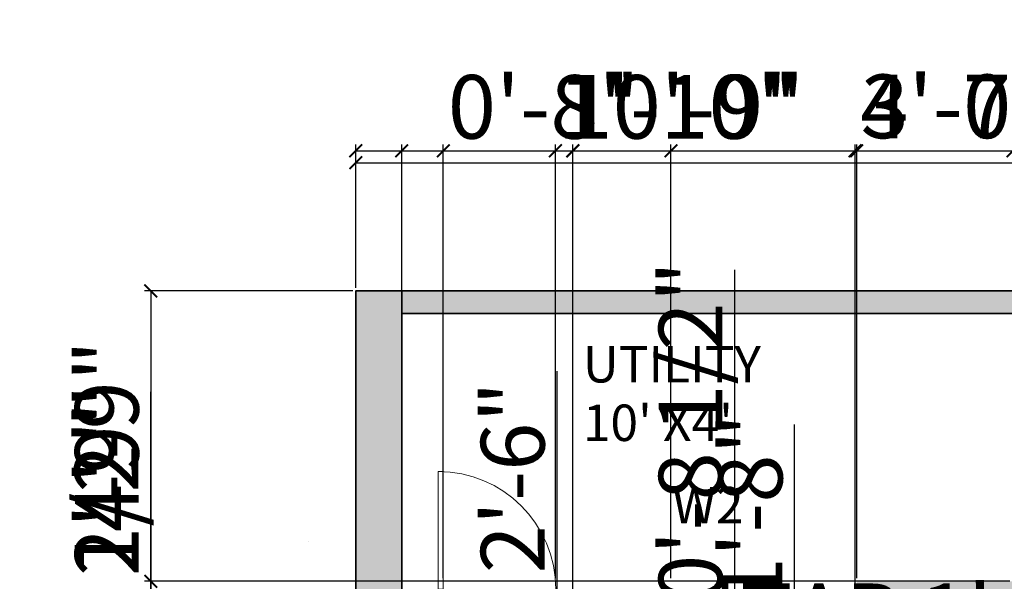
# Model space of a CAD drawing. Units: inches. Extents: x 1763 to 2368, y 1500 to 2097.
# Tile 9 of 24: x 1763 to 1956, y 1986 to 2097. Entities that reach past the tile are written whole.
import ezdxf

# ---------------------------------------------------------------- set-up
doc = ezdxf.new("R2010")
doc.units = ezdxf.units.IN
for name, color, linetype, lineweight in [('A-ANNO-DIMS', 2, 'Continuous', 18), ('A-ANNO-TEXT', 7, 'Continuous', 18), ('A-AREA-IDEN', 7, 'Continuous', 18), ('A-DOOR', 4, 'Continuous', 18), ('A-DRAF-AIDE', 8, 'Continuous', 13), ('A-WALL', 7, 'Continuous', 35), ('A-WALL-PATT', 7, 'Continuous', 13)]:
    doc.layers.add(name, color=color, linetype=linetype, lineweight=lineweight)
doc.styles.get("Standard").update_dxf_attribs({"font": 'arial.ttf'})
doc.dimstyles.new('ISO-25', dxfattribs={"dimtxt": 12.5, "dimasz": 2.5, "dimexe": 1.25, "dimexo": 0.625, "dimtad": 1, "dimdec": 0, "dimlunit": 4, "dimtxsty": 'Standard', "dimblk": 'ARCHTICK', "dimcen": 2.5, "dimclrd": 3, "dimclrt": 4, "dimadec": 0, "dimazin": 0, "dimtfac": 1, "dimtdec": 0, "dimtmove": 0, "dimatfit": 3, "dimfxl": 1, "dimarcsym": 0})

# ---------------------------------------------------------------- blocks, each defined once
blk = doc.blocks.new('*U3')
for p, q in [((0, 0), (0, -6)), ((40, 0), (40, -6))]:
    blk.add_line(p, q)
blk.add_lwpolyline([(0, 0), (0, 40), (1.75, 40), (1.75, 0)], close=True)
blk.add_arc((0, 0), 40, 0, 90)
blk = doc.blocks.new('_ArchTick')
at = {"color": 0, "linetype": 'ByBlock', "const_width": 0.15}
blk.add_lwpolyline([(-0.5, -0.5), (0.5, 0.5)], dxfattribs=at)
blk = doc.blocks.new('*D21')
at = {"layer": 'A-ANNO-DIMS', "color": 0, "lineweight": -2, "transparency": 16777216}
for p, q in [((1829.09, 2043.9), (1829.09, 2069.68)), ((2189.09, 2043.9), (2189.09, 2069.68)), ((1829.09, 2068.43), (2189.09, 2068.43))]:
    blk.add_line(p, q, dxfattribs=at)
at = {"layer": 'Defpoints', "color": 0, "transparency": 16777216}
for p in [(2189.09, 2068.43), (1829.09, 2043.27), (2189.09, 2043.27)]:
    blk.add_point(p, dxfattribs=at)
at = {"layer": 'A-ANNO-DIMS', "color": 0, "lineweight": -2, "transparency": 16777216, "xscale": 2.5, "yscale": 2.5, "zscale": 2.5, "rotation": 180}
blk.add_blockref('_ArchTick', (1829.09, 2068.43), dxfattribs=at)
at = {"layer": 'A-ANNO-DIMS', "color": 0, "lineweight": -2, "transparency": 16777216, "xscale": 2.5, "yscale": 2.5, "zscale": 2.5}
blk.add_blockref('_ArchTick', (2189.09, 2068.43), dxfattribs=at)
at = {"layer": 'A-ANNO-DIMS', "color": 0, "transparency": 16777216, "insert": (2009.09, 2075.45), "char_height": 12.5, "attachment_point": 5}
blk.add_mtext("30'", dxfattribs=at)
blk = doc.blocks.new('*D29')
at = {"layer": 'A-ANNO-DIMS', "color": 3, "lineweight": -2, "transparency": 16777216}
for p, q in [((1868.59, 1924.21), (1868.59, 2027.49)), ((1868.59, 1894.21), (1868.59, 1924.21))]:
    blk.add_line(p, q, dxfattribs=at)
at = {"layer": 'A-ANNO-DIMS', "color": 0, "lineweight": -2, "transparency": 16777216}
for p, q in [((1864.72, 1924.21), (1869.84, 1924.21)), ((1864.72, 1894.21), (1869.84, 1894.21))]:
    blk.add_line(p, q, dxfattribs=at)
at = {"layer": 'Defpoints', "color": 0, "transparency": 16777216}
for p in [(1864.09, 1924.21), (1868.59, 1924.21), (1864.09, 1894.21)]:
    blk.add_point(p, dxfattribs=at)
at = {"layer": 'A-ANNO-DIMS', "color": 3, "lineweight": -2, "transparency": 16777216, "xscale": 2.5, "yscale": 2.5, "zscale": 2.5}
for p, rotation in [((1868.59, 1924.21), 90), ((1868.59, 1894.21), 270)]:
    blk.add_blockref('_ArchTick', p, dxfattribs=dict(at, rotation=rotation))
at = {"layer": 'A-ANNO-DIMS', "color": 4, "transparency": 16777216, "insert": (1861.5, 1977.1), "char_height": 12.5, "attachment_point": 5, "rotation": 90}
blk.add_mtext('RANGE 2\'-6"', dxfattribs=at)
blk = doc.blocks.new('*D32')
at = {"layer": 'A-ANNO-DIMS', "color": 3, "lineweight": -2, "transparency": 16777216}
for p, q in [((1915.18, 1981.27), (1915.18, 2017.07)), ((1915.18, 1961.27), (1915.18, 1981.27))]:
    blk.add_line(p, q, dxfattribs=at)
at = {"layer": 'A-ANNO-DIMS', "color": 0, "lineweight": -2, "transparency": 16777216}
for p, q in [((1911.31, 1981.27), (1916.43, 1981.27)), ((1911.31, 1961.27), (1916.43, 1961.27))]:
    blk.add_line(p, q, dxfattribs=at)
at = {"layer": 'Defpoints', "color": 0, "transparency": 16777216}
for p in [(1910.68, 1981.27), (1915.18, 1981.27), (1910.68, 1961.27)]:
    blk.add_point(p, dxfattribs=at)
at = {"layer": 'A-ANNO-DIMS', "color": 3, "lineweight": -2, "transparency": 16777216, "xscale": 2.5, "yscale": 2.5, "zscale": 2.5}
for p, rotation in [((1915.18, 1981.27), 90), ((1915.18, 1961.27), 270)]:
    blk.add_blockref('_ArchTick', p, dxfattribs=dict(at, rotation=rotation))
at = {"layer": 'A-ANNO-DIMS', "color": 4, "transparency": 16777216, "insert": (1908.18, 2000.42), "char_height": 12.5, "attachment_point": 5, "rotation": 90}
blk.add_mtext('1\'-8"', dxfattribs=at)
blk = doc.blocks.new('*D35')
at = {"layer": 'A-ANNO-DIMS', "color": 0, "lineweight": -2, "transparency": 16777216}
for p, q in [((1889.68, 1972.15), (1889.68, 1969.72)), ((1901.68, 1972.15), (1901.68, 1969.72))]:
    blk.add_line(p, q, dxfattribs=at)
at = {"layer": 'A-ANNO-DIMS', "color": 3, "lineweight": -2, "transparency": 16777216}
for p, q in [((1889.68, 1970.97), (1901.68, 1970.97)), ((1901.68, 1970.97), (1977.79, 1970.97))]:
    blk.add_line(p, q, dxfattribs=at)
at = {"layer": 'Defpoints', "color": 0, "transparency": 16777216}
for p in [(1889.68, 1972.77), (1901.68, 1972.77), (1901.68, 1970.97)]:
    blk.add_point(p, dxfattribs=at)
at = {"layer": 'A-ANNO-DIMS', "color": 3, "lineweight": -2, "transparency": 16777216, "xscale": 2.5, "yscale": 2.5, "zscale": 2.5, "rotation": 180}
blk.add_blockref('_ArchTick', (1889.68, 1970.97), dxfattribs=at)
at = {"layer": 'A-ANNO-DIMS', "color": 3, "lineweight": -2, "transparency": 16777216, "xscale": 2.5, "yscale": 2.5, "zscale": 2.5}
blk.add_blockref('_ArchTick', (1901.68, 1970.97), dxfattribs=at)
at = {"layer": 'A-ANNO-DIMS', "color": 4, "transparency": 16777216, "insert": (1940.99, 1977.98), "char_height": 12.5, "attachment_point": 5}
blk.add_mtext('TAP 1\'-0"', dxfattribs=at)
blk = doc.blocks.new('*D36')
at = {"layer": 'A-ANNO-DIMS', "color": 3, "lineweight": -2, "transparency": 16777216}
for p, q in [((1903.48, 1981.27), (1903.48, 2047.38)), ((1903.48, 1972.77), (1903.48, 1981.27))]:
    blk.add_line(p, q, dxfattribs=at)
at = {"layer": 'A-ANNO-DIMS', "color": 0, "lineweight": -2, "transparency": 16777216}
for p, q in [((1902.31, 1981.27), (1904.73, 1981.27)), ((1902.31, 1972.77), (1904.73, 1972.77))]:
    blk.add_line(p, q, dxfattribs=at)
at = {"layer": 'Defpoints', "color": 0, "transparency": 16777216}
for p in [(1901.68, 1981.27), (1903.48, 1981.27), (1901.68, 1972.77)]:
    blk.add_point(p, dxfattribs=at)
at = {"layer": 'A-ANNO-DIMS', "color": 3, "lineweight": -2, "transparency": 16777216, "xscale": 2.5, "yscale": 2.5, "zscale": 2.5}
for p, rotation in [((1903.48, 1981.27), 90), ((1903.48, 1972.77), 270)]:
    blk.add_blockref('_ArchTick', p, dxfattribs=dict(at, rotation=rotation))
at = {"layer": 'A-ANNO-DIMS', "color": 4, "transparency": 16777216, "insert": (1896.4, 2015.58), "char_height": 12.5, "attachment_point": 5, "rotation": 90}
blk.add_mtext('0\'-8 1/2"', dxfattribs=at)
blk = doc.blocks.new('*D44')
at = {"layer": 'A-ANNO-DIMS', "color": 0, "lineweight": -2, "transparency": 16777216}
for p, q in [((1828.47, 2043.27), (1787.6, 2043.27)), ((1837.47, 1986.27), (1787.6, 1986.27))]:
    blk.add_line(p, q, dxfattribs=at)
at = {"layer": 'A-ANNO-DIMS', "color": 3, "lineweight": -2, "transparency": 16777216}
blk.add_line((1788.85, 2043.27), (1788.85, 1986.27), dxfattribs=at)
at = {"layer": 'Defpoints', "color": 0, "transparency": 16777216}
for p in [(1829.09, 2043.27), (1788.85, 1986.27), (1838.09, 1986.27)]:
    blk.add_point(p, dxfattribs=at)
at = {"layer": 'A-ANNO-DIMS', "color": 3, "lineweight": -2, "transparency": 16777216, "xscale": 2.5, "yscale": 2.5, "zscale": 2.5}
for p, rotation in [((1788.85, 2043.27), 90), ((1788.85, 1986.27), 270)]:
    blk.add_blockref('_ArchTick', p, dxfattribs=dict(at, rotation=rotation))
at = {"layer": 'A-ANNO-DIMS', "color": 4, "transparency": 16777216, "insert": (1781.85, 2014.77), "char_height": 12.5, "attachment_point": 5, "rotation": 90}
blk.add_mtext('4\'-9"', dxfattribs=at)
blk = doc.blocks.new('*D50')
at = {"layer": 'A-ANNO-DIMS', "color": 3, "lineweight": -2, "transparency": 16777216}
for p, q in [((1788.85, 1953.39), (1788.85, 2019.48)), ((1788.85, 1913.1), (1788.85, 1953.39))]:
    blk.add_line(p, q, dxfattribs=at)
at = {"layer": 'A-ANNO-DIMS', "color": 0, "lineweight": -2, "transparency": 16777216}
for p, q in [((1828.47, 1953.39), (1787.6, 1953.39)), ((1828.47, 1913.1), (1787.6, 1913.1))]:
    blk.add_line(p, q, dxfattribs=at)
at = {"layer": 'Defpoints', "color": 0, "transparency": 16777216}
for p in [(1788.85, 1953.39), (1829.09, 1953.39), (1829.09, 1913.1)]:
    blk.add_point(p, dxfattribs=at)
at = {"layer": 'A-ANNO-DIMS', "color": 3, "lineweight": -2, "transparency": 16777216, "xscale": 2.5, "yscale": 2.5, "zscale": 2.5}
for p, rotation in [((1788.85, 1953.39), 90), ((1788.85, 1913.1), 270)]:
    blk.add_blockref('_ArchTick', p, dxfattribs=dict(at, rotation=rotation))
at = {"layer": 'A-ANNO-DIMS', "color": 4, "transparency": 16777216, "insert": (1781.76, 1987.69), "char_height": 12.5, "attachment_point": 5, "rotation": 90}
blk.add_mtext('3\'-4 1/2"', dxfattribs=at)
blk = doc.blocks.new('*D51')
at = {"layer": 'A-ANNO-DIMS', "color": 3, "lineweight": -2, "transparency": 16777216}
for p, q in [((1788.85, 1986.27), (1788.85, 2023.46)), ((1788.85, 1953.39), (1788.85, 1986.27))]:
    blk.add_line(p, q, dxfattribs=at)
at = {"layer": 'A-ANNO-DIMS', "color": 0, "lineweight": -2, "transparency": 16777216}
for p, q in [((1837.47, 1986.27), (1787.6, 1986.27)), ((1828.47, 1953.39), (1787.6, 1953.39))]:
    blk.add_line(p, q, dxfattribs=at)
at = {"layer": 'Defpoints', "color": 0, "transparency": 16777216}
for p in [(1788.85, 1986.27), (1838.09, 1986.27), (1829.09, 1953.39)]:
    blk.add_point(p, dxfattribs=at)
at = {"layer": 'A-ANNO-DIMS', "color": 3, "lineweight": -2, "transparency": 16777216, "xscale": 2.5, "yscale": 2.5, "zscale": 2.5}
for p, rotation in [((1788.85, 1986.27), 90), ((1788.85, 1953.39), 270)]:
    blk.add_blockref('_ArchTick', p, dxfattribs=dict(at, rotation=rotation))
at = {"layer": 'A-ANNO-DIMS', "color": 4, "transparency": 16777216, "insert": (1781.85, 2006.12), "char_height": 12.5, "attachment_point": 5, "rotation": 90}
blk.add_mtext('2\'-9"', dxfattribs=at)
blk = doc.blocks.new('*D58')
at = {"layer": 'A-ANNO-DIMS', "color": 0, "lineweight": -2, "transparency": 16777216}
for p, q in [((1871.68, 1635.9), (1871.68, 2072.02)), ((1927.07, 1635.9), (1927.07, 2072.02))]:
    blk.add_line(p, q, dxfattribs=at)
at = {"layer": 'A-ANNO-DIMS', "color": 3, "lineweight": -2, "transparency": 16777216}
for p, q in [((1871.68, 2070.77), (1927.07, 2070.77)), ((1927.07, 2070.77), (1993.68, 2070.77))]:
    blk.add_line(p, q, dxfattribs=at)
at = {"layer": 'Defpoints', "color": 0, "transparency": 16777216}
for p in [(1927.07, 2070.77), (1871.68, 1635.27), (1927.07, 1635.27)]:
    blk.add_point(p, dxfattribs=at)
at = {"layer": 'A-ANNO-DIMS', "color": 3, "lineweight": -2, "transparency": 16777216, "xscale": 2.5, "yscale": 2.5, "zscale": 2.5, "rotation": 180}
blk.add_blockref('_ArchTick', (1871.68, 2070.77), dxfattribs=at)
at = {"layer": 'A-ANNO-DIMS', "color": 3, "lineweight": -2, "transparency": 16777216, "xscale": 2.5, "yscale": 2.5, "zscale": 2.5}
blk.add_blockref('_ArchTick', (1927.07, 2070.77), dxfattribs=at)
at = {"layer": 'A-ANNO-DIMS', "color": 4, "transparency": 16777216, "insert": (1961.63, 2077.86), "char_height": 12.5, "attachment_point": 5}
blk.add_mtext('4\'-7 1/2"', dxfattribs=at)
blk = doc.blocks.new('*D64')
at = {"layer": 'A-ANNO-DIMS', "color": 0, "lineweight": -2, "transparency": 16777216}
for p, q in [((1838.09, 1986.9), (1838.09, 2072.02)), ((1846.24, 1986.9), (1846.24, 2072.02))]:
    blk.add_line(p, q, dxfattribs=at)
at = {"layer": 'A-ANNO-DIMS', "color": 3, "lineweight": -2, "transparency": 16777216}
for p, q in [((1838.09, 2070.77), (1846.24, 2070.77)), ((1846.24, 2070.77), (1883.21, 2070.77))]:
    blk.add_line(p, q, dxfattribs=at)
at = {"layer": 'Defpoints', "color": 0, "transparency": 16777216}
for p in [(1846.24, 2070.77), (1838.09, 1986.27), (1846.24, 1986.27)]:
    blk.add_point(p, dxfattribs=at)
at = {"layer": 'A-ANNO-DIMS', "color": 3, "lineweight": -2, "transparency": 16777216, "xscale": 2.5, "yscale": 2.5, "zscale": 2.5, "rotation": 180}
blk.add_blockref('_ArchTick', (1838.09, 2070.77), dxfattribs=at)
at = {"layer": 'A-ANNO-DIMS', "color": 3, "lineweight": -2, "transparency": 16777216, "xscale": 2.5, "yscale": 2.5, "zscale": 2.5}
blk.add_blockref('_ArchTick', (1846.24, 2070.77), dxfattribs=at)
at = {"layer": 'A-ANNO-DIMS', "color": 4, "transparency": 16777216, "insert": (1865.97, 2077.78), "char_height": 12.5, "attachment_point": 5}
blk.add_mtext('0\'-8"', dxfattribs=at)
blk = doc.blocks.new('*D65')
at = {"layer": 'A-ANNO-DIMS', "color": 0, "lineweight": -2, "transparency": 16777216}
for p, q in [((1846.24, 1986.9), (1846.24, 2072.02)), ((1868.27, 1986.9), (1868.27, 2072.02))]:
    blk.add_line(p, q, dxfattribs=at)
at = {"layer": 'A-ANNO-DIMS', "color": 3, "lineweight": -2, "transparency": 16777216}
for p, q in [((1846.24, 2070.77), (1868.27, 2070.77)), ((1868.27, 2070.77), (1913.79, 2070.77))]:
    blk.add_line(p, q, dxfattribs=at)
at = {"layer": 'Defpoints', "color": 0, "transparency": 16777216}
for p in [(1868.27, 2070.77), (1846.24, 1986.27), (1868.27, 1986.27)]:
    blk.add_point(p, dxfattribs=at)
at = {"layer": 'A-ANNO-DIMS', "color": 3, "lineweight": -2, "transparency": 16777216, "xscale": 2.5, "yscale": 2.5, "zscale": 2.5, "rotation": 180}
blk.add_blockref('_ArchTick', (1846.24, 2070.77), dxfattribs=at)
at = {"layer": 'A-ANNO-DIMS', "color": 3, "lineweight": -2, "transparency": 16777216, "xscale": 2.5, "yscale": 2.5, "zscale": 2.5}
blk.add_blockref('_ArchTick', (1868.27, 2070.77), dxfattribs=at)
at = {"layer": 'A-ANNO-DIMS', "color": 4, "transparency": 16777216, "insert": (1892.28, 2077.78), "char_height": 12.5, "attachment_point": 5}
blk.add_mtext('1\'-10"', dxfattribs=at)
blk = doc.blocks.new('*D66')
at = {"layer": 'A-ANNO-DIMS', "color": 0, "lineweight": -2, "transparency": 16777216}
for p, q in [((1927.39, 1986.9), (1927.39, 2072.02)), ((1958.09, 1986.9), (1958.09, 2072.02))]:
    blk.add_line(p, q, dxfattribs=at)
at = {"layer": 'A-ANNO-DIMS', "color": 3, "lineweight": -2, "transparency": 16777216}
for p, q in [((1927.39, 2070.77), (1958.09, 2070.77)), ((1958.09, 2070.77), (2024.41, 2070.77))]:
    blk.add_line(p, q, dxfattribs=at)
at = {"layer": 'Defpoints', "color": 0, "transparency": 16777216}
for p in [(1958.09, 2070.77), (1927.39, 1986.27), (1958.09, 1986.27)]:
    blk.add_point(p, dxfattribs=at)
at = {"layer": 'A-ANNO-DIMS', "color": 3, "lineweight": -2, "transparency": 16777216, "xscale": 2.5, "yscale": 2.5, "zscale": 2.5, "rotation": 180}
blk.add_blockref('_ArchTick', (1927.39, 2070.77), dxfattribs=at)
at = {"layer": 'A-ANNO-DIMS', "color": 3, "lineweight": -2, "transparency": 16777216, "xscale": 2.5, "yscale": 2.5, "zscale": 2.5}
blk.add_blockref('_ArchTick', (1958.09, 2070.77), dxfattribs=at)
at = {"layer": 'A-ANNO-DIMS', "color": 4, "transparency": 16777216, "insert": (1992.5, 2077.86), "char_height": 12.5, "attachment_point": 5}
blk.add_mtext('2\'-6 1/2"', dxfattribs=at)
blk = doc.blocks.new('*D67')
at = {"layer": 'A-ANNO-DIMS', "color": 0, "lineweight": -2, "transparency": 16777216}
for p, q in [((1890.93, 1986.9), (1890.93, 2072.02)), ((1927.39, 1986.9), (1927.39, 2072.02))]:
    blk.add_line(p, q, dxfattribs=at)
at = {"layer": 'A-ANNO-DIMS', "color": 3, "lineweight": -2, "transparency": 16777216}
for p, q in [((1890.93, 2070.77), (1927.39, 2070.77)), ((1927.39, 2070.77), (1993.49, 2070.77))]:
    blk.add_line(p, q, dxfattribs=at)
at = {"layer": 'Defpoints', "color": 0, "transparency": 16777216}
for p in [(1927.39, 2070.77), (1890.93, 1986.27), (1927.39, 1986.27)]:
    blk.add_point(p, dxfattribs=at)
at = {"layer": 'A-ANNO-DIMS', "color": 3, "lineweight": -2, "transparency": 16777216, "xscale": 2.5, "yscale": 2.5, "zscale": 2.5, "rotation": 180}
blk.add_blockref('_ArchTick', (1890.93, 2070.77), dxfattribs=at)
at = {"layer": 'A-ANNO-DIMS', "color": 3, "lineweight": -2, "transparency": 16777216, "xscale": 2.5, "yscale": 2.5, "zscale": 2.5}
blk.add_blockref('_ArchTick', (1927.39, 2070.77), dxfattribs=at)
at = {"layer": 'A-ANNO-DIMS', "color": 4, "transparency": 16777216, "insert": (1961.69, 2077.87), "char_height": 12.5, "attachment_point": 5}
blk.add_mtext('3\'-0 1/2"', dxfattribs=at)
blk = doc.blocks.new('*D84')
at = {"layer": 'A-ANNO-DIMS', "color": 0, "lineweight": -2, "transparency": 16777216}
for p, q in [((1829.09, 2043.9), (1829.09, 2072.02)), ((1958.09, 2039.45), (1958.09, 2072.02))]:
    blk.add_line(p, q, dxfattribs=at)
at = {"layer": 'A-ANNO-DIMS', "color": 3, "lineweight": -2, "transparency": 16777216}
blk.add_line((1829.09, 2070.77), (1958.09, 2070.77), dxfattribs=at)
at = {"layer": 'Defpoints', "color": 0, "transparency": 16777216}
for p in [(1958.09, 2070.77), (1829.09, 2043.27), (1958.09, 2038.83)]:
    blk.add_point(p, dxfattribs=at)
at = {"layer": 'A-ANNO-DIMS', "color": 3, "lineweight": -2, "transparency": 16777216, "xscale": 2.5, "yscale": 2.5, "zscale": 2.5, "rotation": 180}
blk.add_blockref('_ArchTick', (1829.09, 2070.77), dxfattribs=at)
at = {"layer": 'A-ANNO-DIMS', "color": 3, "lineweight": -2, "transparency": 16777216, "xscale": 2.5, "yscale": 2.5, "zscale": 2.5}
blk.add_blockref('_ArchTick', (1958.09, 2070.77), dxfattribs=at)
at = {"layer": 'A-ANNO-DIMS', "color": 4, "transparency": 16777216, "insert": (1893.59, 2077.78), "char_height": 12.5, "attachment_point": 5}
blk.add_mtext('10\'-9"', dxfattribs=at)
blk = doc.blocks.new('*D85')
at = {"layer": 'A-ANNO-DIMS', "color": 0, "lineweight": -2, "transparency": 16777216}
for p, q in [((1957.47, 1986.27), (1787.6, 1986.27)), ((1958.51, 1880.27), (1787.6, 1880.27))]:
    blk.add_line(p, q, dxfattribs=at)
at = {"layer": 'A-ANNO-DIMS', "color": 3, "lineweight": -2, "transparency": 16777216}
blk.add_line((1788.85, 1986.27), (1788.85, 1880.27), dxfattribs=at)
at = {"layer": 'Defpoints', "color": 0, "transparency": 16777216}
for p in [(1958.09, 1986.27), (1788.85, 1880.27), (1959.13, 1880.27)]:
    blk.add_point(p, dxfattribs=at)
at = {"layer": 'A-ANNO-DIMS', "color": 3, "lineweight": -2, "transparency": 16777216, "xscale": 2.5, "yscale": 2.5, "zscale": 2.5}
for p, rotation in [((1788.85, 1986.27), 90), ((1788.85, 1880.27), 270)]:
    blk.add_blockref('_ArchTick', p, dxfattribs=dict(at, rotation=rotation))
at = {"layer": 'A-ANNO-DIMS', "color": 4, "transparency": 16777216, "insert": (1781.85, 1933.27), "char_height": 12.5, "attachment_point": 5, "rotation": 90}
blk.add_mtext('8\'-10"', dxfattribs=at)

msp = doc.modelspace()

# ---------------------------------------------------------------- hatches: boundary and pattern name
at = {"layer": 'A-WALL-PATT'}
h = msp.add_hatch(color=256, dxfattribs=at)
h.dxf.hatch_style = 1
h.paths.add_polyline_path([(1838.09, 2034.27), (1838.09, 2043.27), (1829.09, 2043.27), (1829.09, 1953.39), (1838.09, 1953.39)])
h.paths.add_polyline_path([(1838.09, 1913.1), (1829.09, 1913.1), (1829.09, 1862.2), (1838.09, 1862.2)])
h.paths.add_polyline_path([(1838.09, 1825.59), (1829.09, 1825.59), (1829.09, 1738.64), (1838.09, 1738.64)])
h.paths.add_polyline_path([(1895.59, 1885.27), (1838.09, 1885.27), (1838.09, 1880.27), (1895.59, 1880.27)])
h.paths.add_polyline_path([(1857.39, 1784.27), (1838.09, 1784.27), (1838.09, 1779.27), (1857.39, 1779.27)])
h.paths.add_polyline_path([(1958.09, 1981.27), (1971.46, 1981.27), (1971.46, 1986.27), (1968.57, 1986.27), (1958.09, 1986.27), (1953.09, 1986.27), (1927.39, 1986.27), (1927.39, 1981.27), (1953.09, 1981.27), (1953.09, 1885.27), (1932.01, 1885.27), (1932.01, 1880.27), (1959.13, 1880.27), (1959.13, 1883.74), (1959.13, 1885.27), (1958.09, 1885.27)])
h.paths.add_polyline_path([(2018.09, 1981.27), (2031.02, 1981.27), (2031.02, 1986.27), (2018.09, 1986.27), (2013.09, 1986.27), (2001.23, 1986.27), (2001.23, 1981.27), (2013.09, 1981.27), (2013.09, 1885.27), (1982.18, 1885.27, -0.016629), (1982.23, 1883.74), (1982.23, 1880.27), (2049.69, 1880.27), (2049.69, 1883.74, -0.016629), (2049.74, 1885.27), (2018.09, 1885.27)])
h.paths.add_polyline_path([(2083.09, 1981.27), (2120.61, 1981.27), (2120.61, 1986.27), (2083.09, 1986.27), (2078.09, 1986.27), (2063.14, 1986.27), (2063.14, 1981.27), (2078.09, 1981.27), (2078.09, 1885.27), (2072.78, 1885.27), (2072.78, 1883.74), (2072.78, 1880.27), (2078.09, 1880.27), (2078.09, 1866.87), (2081.56, 1866.87, -0.016629), (2083.09, 1866.82)])
h.paths.add_polyline_path([(1871.68, 1635.27), (1838.09, 1635.27), (1838.09, 1626.27), (1871.68, 1626.27)], flags=17)
h.paths.add_polyline_path([(2100.58, 1688.27), (2060.09, 1688.27), (2060.09, 1679.27), (2100.58, 1679.27)], flags=17)
h.paths.add_polyline_path([(2180.09, 1688.27), (2148.74, 1688.27), (2148.74, 1679.27), (2180.09, 1679.27)], flags=17)
h.paths.add_polyline_path([(2189.09, 1746.22), (2180.09, 1746.22), (2180.09, 1743.42), (2180.12, 1743.42), (2180.12, 1726.72), (2180.09, 1572.27), (2034.91, 1572.27), (2034.91, 1565.6), (2034.91, 1563.27), (2189.09, 1563.27)])
h.paths.add_polyline_path([(2060.09, 1802.35, -0.016629), (2058.56, 1802.3), (2055.09, 1802.3), (2055.09, 1635.27), (2042.48, 1635.27), (2042.48, 1629.74), (2042.48, 1626.27), (2055.09, 1626.27), (2055.09, 1599.27), (2040.27, 1599.27), (2040.27, 1590.27), (2060.09, 1590.27)])
h.paths.add_polyline_path([(2019.39, 1629.74, -0.060569), (2020.06, 1635.27), (1995.09, 1635.27), (1990.09, 1635.27), (1927.07, 1635.27), (1927.07, 1626.27), (1990.09, 1626.27), (1990.09, 1590.27), (1995.09, 1590.27), (2005.2, 1590.27), (2005.2, 1599.27), (1995.09, 1599.27), (1995.09, 1626.27), (2019.39, 1626.27)])
edge = h.paths.add_edge_path()
edge.add_line((2180.09, 1837.27), (2167.2, 1837.27))
edge.add_spline(control_points=[(2167.2, 1837.27), (2167.19, 1837.27), (2167.18, 1837.27), (2167.18, 1837.27)], knot_values=[168.955493, 168.955493, 168.955493, 168.955493, 169.065871, 169.065871, 169.065871, 169.065871], degree=3, periodic=0)
edge.add_spline(control_points=[(2167.18, 1837.27), (2166.56, 1837.38), (2166.33, 1846.16), (2165.71, 1846.24)], knot_values=[159.864705, 159.864705, 159.864705, 159.864705, 168.955493, 168.955493, 168.955493, 168.955493], degree=3, periodic=0)
edge.add_line((2167.12, 1837.27), (2163.16, 1837.27))
edge.add_spline(control_points=[(2163.16, 1837.27), (2163.16, 1837.27), (2163.16, 1837.27), (2163.15, 1837.27)], knot_values=[150.537172, 150.537172, 150.537172, 150.537172, 150.553797, 150.553797, 150.553797, 150.553797], degree=3, periodic=0)
edge.add_spline(control_points=[(2163.15, 1837.27), (2162.29, 1837.29), (2161.59, 1846.23), (2160.88, 1846.24)], knot_values=[141.293426, 141.293426, 141.293426, 141.293426, 150.537172, 150.537172, 150.537172, 150.537172], degree=3, periodic=0)
edge.add_line((2163.08, 1837.27), (2158.7, 1837.27))
edge.add_spline(control_points=[(2158.7, 1837.27), (2158.7, 1837.27), (2158.7, 1837.27), (2158.7, 1837.27)], knot_values=[132.033544, 132.033544, 132.033544, 132.033544, 132.049151, 132.049151, 132.049151, 132.049151], degree=3, periodic=0)
edge.add_spline(control_points=[(2158.7, 1837.27), (2157.97, 1837.29), (2157.26, 1846.23), (2156.39, 1846.24)], knot_values=[122.786021, 122.786021, 122.786021, 122.786021, 132.033544, 132.033544, 132.033544, 132.033544], degree=3, periodic=0)
edge.add_line((2158.63, 1837.27), (2153.84, 1837.27))
edge.add_spline(control_points=[(2153.84, 1837.27), (2153.83, 1837.27), (2153.82, 1837.27), (2153.82, 1837.27)], knot_values=[113.451585, 113.451585, 113.451585, 113.451585, 113.562103, 113.562103, 113.562103, 113.562103], degree=3, periodic=0)
edge.add_spline(control_points=[(2153.82, 1837.27), (2153.17, 1837.38), (2152.88, 1846.19), (2152.4, 1846.24)], knot_values=[0, 0, 0, 0, 9.081854, 9.081854, 9.081854, 9.081854], degree=3, periodic=0)
edge.add_line((2153.76, 1837.27), (2150.39, 1837.27))
edge.add_spline(control_points=[(2150.39, 1837.27), (2150.38, 1837.27), (2150.37, 1837.27), (2150.36, 1837.27)], knot_values=[95.069382, 95.069382, 95.069382, 95.069382, 95.17519, 95.17519, 95.17519, 95.17519], degree=3, periodic=0)
edge.add_spline(control_points=[(2150.36, 1837.27), (2149.49, 1837.37), (2148.42, 1846.19), (2147.59, 1846.24)], knot_values=[85.824599, 85.824599, 85.824599, 85.824599, 95.069382, 95.069382, 95.069382, 95.069382], degree=3, periodic=0)
edge.add_line((2150.29, 1837.27), (2145.43, 1837.27))
edge.add_spline(control_points=[(2145.43, 1837.27), (2145.43, 1837.27), (2145.42, 1837.27), (2145.42, 1837.27)], knot_values=[76.505559, 76.505559, 76.505559, 76.505559, 76.547811, 76.547811, 76.547811, 76.547811], degree=3, periodic=0)
edge.add_spline(control_points=[(2145.42, 1837.27), (2144.68, 1837.31), (2143.8, 1846.19), (2142.95, 1846.24)], knot_values=[67.23945, 67.23945, 67.23945, 67.23945, 76.505559, 76.505559, 76.505559, 76.505559], degree=3, periodic=0)
edge.add_line((2145.35, 1837.27), (2134.57, 1837.27))
edge.add_spline(control_points=[(2134.57, 1837.27), (2134.57, 1837.27), (2134.56, 1837.27), (2134.56, 1837.27)], knot_values=[39.001463, 39.001463, 39.001463, 39.001463, 39.045107, 39.045107, 39.045107, 39.045107], degree=3, periodic=0)
edge.add_spline(control_points=[(2134.56, 1837.27), (2133.87, 1837.31), (2133.4, 1845.85), (2132.33, 1846.24)], knot_values=[29.79778, 29.79778, 29.79778, 29.79778, 39.001463, 39.001463, 39.001463, 39.001463], degree=3, periodic=0)
edge.add_line((2134.5, 1837.27), (2128.08, 1837.27))
edge.add_spline(control_points=[(2128.08, 1837.27), (2128.03, 1837.26), (2127.98, 1837.26), (2127.93, 1837.27)], knot_values=[19.482067, 19.482067, 19.482067, 19.482067, 19.869396, 19.869396, 19.869396, 19.869396], degree=3, periodic=0)
edge.add_spline(control_points=[(2125.01, 1846.24), (2126.16, 1844.66), (2126.82, 1837.57), (2127.93, 1837.27)], knot_values=[10.389805, 10.389805, 10.389805, 10.389805, 19.482067, 19.482067, 19.482067, 19.482067], degree=3, periodic=0)
edge.add_line((2127.93, 1837.27), (2083.09, 1837.27))
edge.add_line((2083.09, 1837.27), (2083.09, 1843.77))
edge.add_line((2083.09, 1843.77), (2081.56, 1843.77))
edge.add_line((2081.56, 1843.77), (2078.09, 1843.77))
edge.add_line((2078.09, 1843.77), (2078.09, 1837.27))
edge.add_line((2078.09, 1837.27), (2055.09, 1837.27))
edge.add_line((2055.09, 1837.27), (2055.09, 1825.4))
edge.add_line((2055.09, 1825.4), (2058.56, 1825.4))
edge.add_line((2058.56, 1825.4), (2060.09, 1825.4))
edge.add_line((2060.09, 1825.4), (2060.09, 1832.27))
edge.add_line((2060.09, 1832.27), (2122.44, 1832.27))
edge.add_spline(control_points=[(2122.44, 1832.27), (2122.73, 1832.58), (2123.01, 1832.62), (2123.28, 1832.27)], knot_values=[5.972033, 5.972033, 5.972033, 5.972033, 8.057258, 8.057258, 8.057258, 8.057258], degree=3, periodic=0)
edge.add_line((2123.28, 1832.27), (2137.95, 1832.27))
edge.add_spline(control_points=[(2137.95, 1832.27), (2137.96, 1832.27), (2137.97, 1832.27), (2137.98, 1832.27)], knot_values=[53.926862, 53.926862, 53.926862, 53.926862, 54.030075, 54.030075, 54.030075, 54.030075], degree=3, periodic=0)
edge.add_spline(control_points=[(2139.72, 1825.02), (2139.28, 1825.06), (2138.67, 1832.18), (2137.98, 1832.27)], knot_values=[54.030075, 54.030075, 54.030075, 54.030075, 61.445194, 61.445194, 61.445194, 61.445194], degree=3, periodic=0)
edge.add_line((2138.05, 1832.27), (2140.96, 1832.27))
edge.add_spline(control_points=[(2140.96, 1832.27), (2140.97, 1832.27), (2140.98, 1832.27), (2140.99, 1832.27)], knot_values=[68.854182, 68.854182, 68.854182, 68.854182, 68.971237, 68.971237, 68.971237, 68.971237], degree=3, periodic=0)
edge.add_spline(control_points=[(2143.19, 1825.02), (2142.44, 1825.07), (2141.56, 1832.16), (2140.99, 1832.27)], knot_values=[68.971237, 68.971237, 68.971237, 68.971237, 76.444911, 76.444911, 76.444911, 76.444911], degree=3, periodic=0)
edge.add_line((2141.04, 1832.27), (2145.43, 1832.27))
edge.add_spline(control_points=[(2145.43, 1832.27), (2145.44, 1832.27), (2145.45, 1832.27), (2145.46, 1832.27)], knot_values=[84.039047, 84.039047, 84.039047, 84.039047, 84.124041, 84.124041, 84.124041, 84.124041], degree=3, periodic=0)
edge.add_spline(control_points=[(2148.11, 1825.02), (2147.34, 1825.02), (2146.3, 1832.19), (2145.46, 1832.27)], knot_values=[84.124041, 84.124041, 84.124041, 84.124041, 91.773891, 91.773891, 91.773891, 91.773891], degree=3, periodic=0)
edge.add_line((2145.54, 1832.27), (2150.39, 1832.27))
edge.add_spline(control_points=[(2150.39, 1832.27), (2150.42, 1832.28), (2150.45, 1832.28), (2150.47, 1832.27)], knot_values=[99.381577, 99.381577, 99.381577, 99.381577, 99.573457, 99.573457, 99.573457, 99.573457], degree=3, periodic=0)
edge.add_spline(control_points=[(2153.97, 1825.02), (2153.09, 1825.28), (2151.53, 1832.1), (2150.47, 1832.27)], knot_values=[99.573457, 99.573457, 99.573457, 99.573457, 107.218357, 107.218357, 107.218357, 107.218357], degree=3, periodic=0)
edge.add_line((2150.57, 1832.27), (2155.6, 1832.27))
edge.add_spline(control_points=[(2155.6, 1832.27), (2155.6, 1832.27), (2155.61, 1832.27), (2155.62, 1832.27)], knot_values=[114.933058, 114.933058, 114.933058, 114.933058, 115.013624, 115.013624, 115.013624, 115.013624], degree=3, periodic=0)
edge.add_spline(control_points=[(2158.28, 1825.02), (2157.4, 1825.07), (2156.25, 1832.2), (2155.62, 1832.27)], knot_values=[115.013624, 115.013624, 115.013624, 115.013624, 122.616269, 122.616269, 122.616269, 122.616269], degree=3, periodic=0)
edge.add_line((2155.68, 1832.27), (2165.19, 1832.27))
edge.add_spline(control_points=[(2165.19, 1832.27), (2165.2, 1832.27), (2165.2, 1832.27), (2165.2, 1832.27)], knot_values=[145.488477, 145.488477, 145.488477, 145.488477, 145.516379, 145.516379, 145.516379, 145.516379], degree=3, periodic=0)
edge.add_spline(control_points=[(2167.45, 1825.02), (2166.96, 1825.02), (2166.06, 1832.25), (2165.2, 1832.27)], knot_values=[145.516379, 145.516379, 145.516379, 145.516379, 153.105469, 153.105469, 153.105469, 153.105469], degree=3, periodic=0)
edge.add_line((2165.29, 1832.27), (2168.93, 1832.27))
edge.add_spline(control_points=[(2168.93, 1832.27), (2168.98, 1832.29), (2169.04, 1832.29), (2169.1, 1832.27)], knot_values=[160.517439, 160.517439, 160.517439, 160.517439, 160.939723, 160.939723, 160.939723, 160.939723], degree=3, periodic=0)
edge.add_spline(control_points=[(2171.09, 1828.64), (2170.35, 1830.37), (2169.62, 1832.09), (2169.1, 1832.27)], knot_values=[160.939723, 160.939723, 160.939723, 160.939723, 164.738835, 164.738835, 164.738835, 164.738835], degree=3, periodic=0)
edge.add_line((2169.1, 1832.27), (2180.09, 1832.27))
edge.add_line((2180.09, 1832.27), (2180.09, 1837.27))
h.paths.add_polyline_path([(2189.09, 1885.52), (2180.09, 1885.52), (2180.09, 1813.32), (2180.12, 1813.32), (2180.12, 1796.62), (2180.12, 1795.26), (2189.09, 1795.26)])
h.paths.add_polyline_path([(2180.09, 1986.27), (2166.28, 1986.27), (2166.28, 1981.27), (2180.09, 1981.27)])
h.paths.add_polyline_path([(2189.09, 2043.27), (2180.09, 2043.27), (2180.09, 2034.27), (2180.09, 1934.11), (2189.09, 1934.11)])
h.paths.add_polyline_path([(1838.09, 1681.59), (1829.09, 1681.59), (1829.09, 1563.27), (2003.86, 1563.27), (2003.86, 1565.6), (2003.86, 1572.27), (1838.09, 1572.27)])
h = msp.add_hatch(color=256, dxfattribs=at)
h.dxf.hatch_style = 1
h.paths.add_polyline_path([(2180.09, 2043.27), (1838.09, 2043.27), (1838.09, 2038.83), (2180.09, 2038.83)])

# ---------------------------------------------------------------- linework, layer by layer
at = {"layer": 'A-DRAF-AIDE'}
msp.add_lwpolyline([(1819.73, 1994.13), (1819.73, 1994.13), (1819.73, 1994.13), (1819.73, 1994.13)], close=True, dxfattribs=at)
at = {"layer": 'A-WALL'}
for p, q in [((1838.09, 2034.27), (1838.09, 2043.27)), ((1838.09, 2043.27), (2180.09, 2043.27)), ((1838.09, 2038.83), (2180.09, 2038.83)), ((1838.09, 1572.27), (1838.09, 2034.27))]:
    msp.add_line(p, q, dxfattribs=at)
msp.add_lwpolyline([(2003.86, 1563.27), (1829.09, 1563.27), (1829.09, 2043.27), (2189.09, 2043.27), (2189.09, 1563.27), (2034.91, 1563.27)], dxfattribs=at)

# ---------------------------------------------------------------- block references
at = {"layer": 'A-DOOR', "xscale": 0.5774759422388936, "yscale": 0.5774759422388936, "zscale": 0.5774759422388936}
msp.add_blockref('*U3', (1845.22, 1984.74), dxfattribs=at)

# ---------------------------------------------------------------- texts
at = {"layer": 'A-ANNO-TEXT'}
msp.add_text('W2', height=7.155, dxfattribs=at).set_placement((1891.19, 1997.65))
at = {"layer": 'A-AREA-IDEN'}
for s, p in [('UTILITY', (1873.64, 2025.3)), ("10' X4'", (1873.64, 2013.81))]:
    msp.add_text(s, height=7.155, dxfattribs=at).set_placement(p)

# ---------------------------------------------------------------- dimensions: what is measured, and where the dimension line sits
at = {"layer": 'A-ANNO-DIMS'}
for base, p1, p2, override, picture, middle in [((1927.07, 2070.77), (1871.68, 1635.27), (1927.07, 1635.27), {"dimdec": 1, "dimlfac": 1, "dimrnd": 0, "dimzin": 1, "dimdsep": 46, "dimlunit": 4, "dimfrac": 2}, '*D58', (1961.63, 2077.86)), ((1927.39, 2070.77), (1890.93, 1986.27), (1927.39, 1986.27), {"dimdec": 1, "dimlfac": 1, "dimrnd": 0, "dimzin": 1, "dimdsep": 46, "dimlunit": 4, "dimfrac": 2}, '*D67', (1961.69, 2077.87)), ((1958.09, 2070.77), (1927.39, 1986.27), (1958.09, 1986.27), {"dimdec": 1, "dimlfac": 1, "dimrnd": 0, "dimzin": 1, "dimdsep": 46, "dimlunit": 4, "dimfrac": 2}, '*D66', (1992.5, 2077.86)), ((1958.09, 2070.77), (1829.09, 2043.27), (1958.09, 2038.83), {"dimdec": 1, "dimlfac": 1, "dimrnd": 0, "dimzin": 1, "dimdsep": 46, "dimlunit": 4, "dimfrac": 2}, '*D84', (1893.59, 2077.78)), ((1846.2352, 2070.7727), (1838.0918, 1986.2727), (1846.2352, 1986.2727), {"dimdec": 1, "dimlfac": 1, "dimrnd": 0, "dimzin": 1, "dimdsep": 46, "dimlunit": 4, "dimfrac": 2}, '*D64', (1865.9743, 2077.7799)), ((1868.27, 2070.77), (1846.24, 1986.27), (1868.27, 1986.27), {"dimdec": 1, "dimlfac": 1, "dimrnd": 0, "dimzin": 1, "dimdsep": 46, "dimlunit": 4, "dimfrac": 2}, '*D65', (1892.28, 2077.78)), ((2189.09, 2068.43), (1829.09, 2043.27), (2189.09, 2043.27), {"dimclrd": 0, "dimclre": 0, "dimclrt": 0}, '*D21', (2009.09, 2075.45))]:
    dim = msp.add_linear_dim(base=base, p1=p1, p2=p2, dimstyle='ISO-25', override=override, dxfattribs=at)
    dim.commit()
    dim.dimension.update_dxf_attribs({"geometry": picture, "text_midpoint": middle})
for base, p1, p2, picture, middle in [((1903.48, 1981.27), (1901.68, 1972.77), (1901.68, 1981.27), '*D36', (1896.4, 2015.58)), ((1788.85, 1986.27), (1829.09, 2043.27), (1838.09, 1986.27), '*D44', (1781.85, 2014.77)), ((1788.85, 1986.27), (1829.09, 1953.39), (1838.09, 1986.27), '*D51', (1781.85, 2006.12)), ((1788.85, 1953.39), (1829.09, 1913.1), (1829.09, 1953.39), '*D50', (1781.76, 1987.69)), ((1915.18, 1981.27), (1910.68, 1961.27), (1910.68, 1981.27), '*D32', (1908.18, 2000.42)), ((1788.85, 1880.27), (1958.09, 1986.27), (1959.13, 1880.27), '*D85', (1781.85, 1933.27))]:
    dim = msp.add_linear_dim(base=base, p1=p1, p2=p2, angle=90, dimstyle='ISO-25', override={"dimdec": 1, "dimlfac": 1, "dimrnd": 0, "dimzin": 1, "dimdsep": 46, "dimlunit": 4, "dimfrac": 2}, dxfattribs=at)
    dim.commit()
    dim.dimension.update_dxf_attribs({"geometry": picture, "text_midpoint": middle})
dim = msp.add_linear_dim(base=(1868.59, 1924.21), p1=(1864.09, 1894.21), p2=(1864.09, 1924.21), angle=90, text='RANGE <>', dimstyle='ISO-25', override={"dimdec": 1, "dimlfac": 1, "dimrnd": 0, "dimzin": 1, "dimdsep": 46, "dimlunit": 4, "dimfrac": 2}, dxfattribs=at)
dim.commit()
dim.dimension.update_dxf_attribs({"geometry": '*D29', "text_midpoint": (1861.5, 1977.1)})
dim = msp.add_linear_dim(base=(1901.68, 1970.97), p1=(1889.68, 1972.77), p2=(1901.68, 1972.77), text='TAP <>', dimstyle='ISO-25', override={"dimdec": 1, "dimlfac": 1, "dimrnd": 0, "dimzin": 1, "dimdsep": 46, "dimlunit": 4, "dimfrac": 2}, dxfattribs=at)
dim.commit()
dim.dimension.update_dxf_attribs({"geometry": '*D35', "text_midpoint": (1940.99, 1977.98)})

doc.saveas('drawing.dxf')
